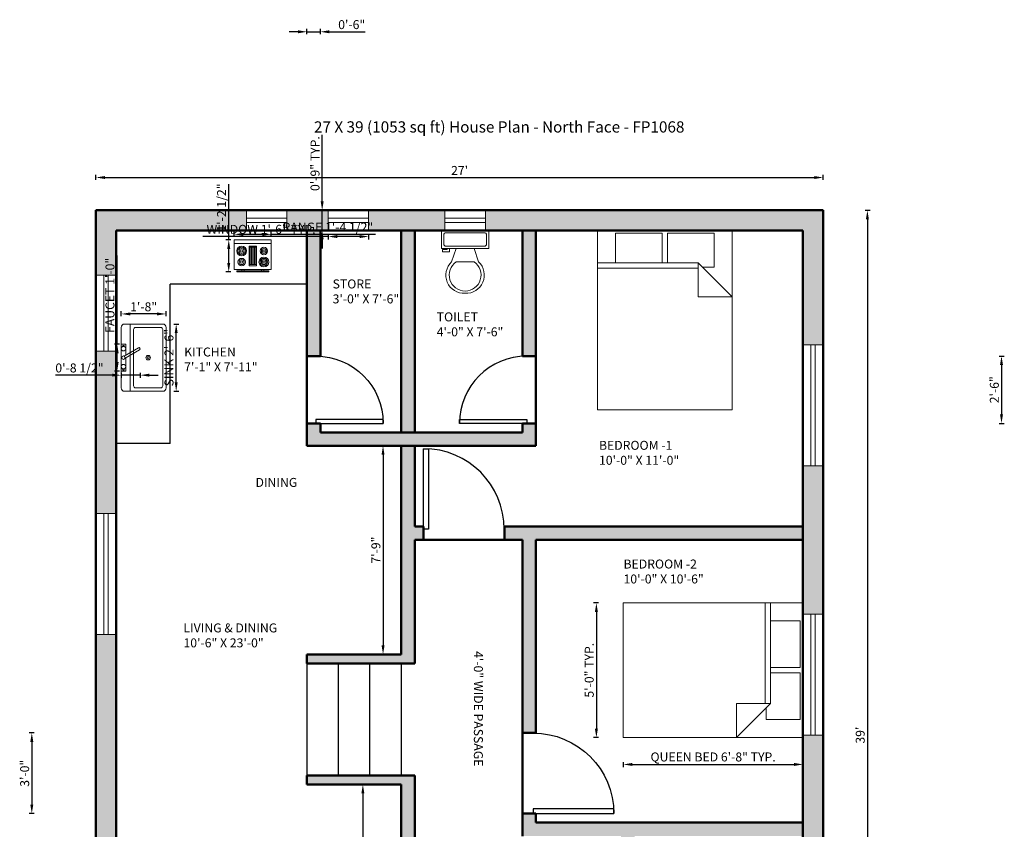
# Model space of a CAD drawing. Units: inches. Extents: x -33 to 405, y -509 to 99.
# Tile 2 of 2: x -33 to 405, y -262 to 99. Entities that reach past the tile are written whole.
import ezdxf

# ---------------------------------------------------------------- set-up
doc = ezdxf.new("R2010")
doc.units = ezdxf.units.IN
for name, color, linetype, lineweight in [('A-ANNO-DIMS', 2, 'Continuous', 18), ('A-ANNO-TEXT', 7, 'Continuous', 25), ('A-AREA-IDEN', 7, 'Continuous', 18), ('A-DOOR', 4, 'Continuous', 25), ('A-EQPM', 8, 'Continuous', 18), ('A-FLOR-CASE', 7, 'Continuous', 25), ('A-FLOR-FIXT', 8, 'Continuous', 18), ('A-FLOR-STRS', 7, 'Continuous', 25), ('A-FURN', 9, 'Continuous', 18), ('A-GLAZ', 6, 'Continuous', 18), ('A-WALL', 7, 'Continuous', 50), ('A-WALL-PATT', 251, 'Continuous', 13)]:
    doc.layers.add(name, color=color, linetype=linetype, lineweight=lineweight)
doc.styles.get("Standard").update_dxf_attribs({"font": 'arial.ttf'})
doc.dimstyles.new('ISO-25', dxfattribs={"dimtxt": 4, "dimasz": 4, "dimexe": 1.25, "dimexo": 0.625, "dimtad": 1, "dimlunit": 3, "dimtxsty": 'Standard', "dimcen": 2.5, "dimadec": 0, "dimazin": 0, "dimtfac": 1, "dimtmove": 0, "dimatfit": 3, "dimfxl": 1, "dimfxlon": 1, "dimarcsym": 0})

# ---------------------------------------------------------------- blocks, each defined once
blk = doc.blocks.new('*U4')
for p, q in [((0, 0), (0, -100)), ((750, 0), (750, -100))]:
    blk.add_line(p, q)
blk.add_lwpolyline([(0, 0), (0, 750), (43.75, 750), (43.75, 0)], close=True)
blk.add_arc((0, 0), 750, 0, 90)
blk = doc.blocks.new('*U2')
for p, q in [((9.5, -6), (9.5, -2)), ((-10, -8.5), (-8, -8.5)), ((-10, -9.5), (-10, -8.5)), ((-8, -8.5), (-8, -8)), ((-7, -8), (-7, -9.5)), ((-4, -8), (-6, -14)), ((4, -8), (6, -14)), ((-7, -9.5), (-10, -9.5)), ((4, -14), (-4, -14))]:
    blk.add_line(p, q)
blk.add_lwpolyline([(10.5, -8), (10.5, 0), (-10.5, 0), (-10.5, -8)], close=True)
for points in [[(-9.5, -2), (-9.5, -6)], [(8.5, -1), (-8.5, -1)], [(-8.5, -7), (8.5, -7)]]:
    blk.add_lwpolyline(points)
for centre, radius, start, end in [((-8.625, -1.875), 0.8839, 81.8699, 188.1301), ((8.625, -1.875), 0.8839, 351.8699, 98.1301), ((-8.625, -6.125), 0.8839, 171.869898, 278.1301), ((8.625, -6.125), 0.8839, 261.8699, 8.1301), ((-0.4772, -19.9188), 8.0953, 133.01722, 273.38), ((0.0374, -19.8731), 7.127, 124.50543, 269.7), ((-0.0373, -19.8731), 7.127, 270.3, 55.4946), ((0.4773, -19.9188), 8.0953, 266.62, 46.9828)]:
    blk.add_arc(centre, radius, start, end)
blk = doc.blocks.new('Sink-single - 30 in top')
blk.add_line((-15, -3.999996), (15, -3.999996))
for points in [[(-13.5, 0), (13.5, 0)], [(-15, -18.499996), (-15, -1.5)], [(15, -1.5), (15, -18.499996)], [(-13.5, -17.499996), (-13.5, -6.499996)], [(-12.5, -5.499996), (12.5, -5.499996)], [(13.5, -6.499996), (13.5, -17.499996)], [(13.5, -19.999996), (-13.5, -19.999996)], [(12.5, -18.499996), (-12.5, -18.499996)]]:
    blk.add_lwpolyline(points)
for radius in [1, 0.5]:
    blk.add_circle((0, -11.999996), radius)
for centre, radius, start, end in [((-13.5, -1.5), 1.5, 90, 180), ((13.5, -1.5), 1.5, 0, 90), ((-12.5, -6.499996), 1, 90, 180), ((12.5, -6.499996), 1, 0, 90), ((-12.5, -17.499996), 1, 180, 270), ((12.5, -17.499996), 1, 270, 0), ((-13.5, -18.499996), 1.5, 180, 270), ((13.5, -18.499996), 1.5, 270, 0)]:
    blk.add_arc(centre, radius, start, end)
blk = doc.blocks.new('Faucet - kit sink top')
for p, q in [((-5.5, -0.75), (-5.5, -1.25)), ((-4.94278, -0.75), (-5.5, -0.75)), ((-5.5, -1.25), (-4.94278, -1.25)), ((-0.14775, -1.7441), (3.56698, -8.1782)), ((4.43301, -7.6782), (0.71828, -1.2441)), ((4.94278, -0.75), (5.5, -0.75)), ((5.5, -1.25), (4.94278, -1.25)), ((5.5, -0.75), (5.5, -1.25))]:
    blk.add_line(p, q)
blk.add_lwpolyline([(-0.00587, -2), (-6, -2), (-6, 0), (6, 0), (6, -2), (1.15195, -2)])
for centre, radius in [((-4, -1), 1), ((4, -1), 1), ((0, -1), 0.75)]:
    blk.add_circle(centre, radius)
blk.add_arc((4, -7.9282), 0.5, 210, 30)
blk = doc.blocks.new('Range-Oven - 30 in top')
for p, q in [((0, -3), (30, -3)), ((12, -6), (18, -6)), ((13, -20), (13, -6)), ((14, -6), (14, -20)), ((15, -20), (15, -6)), ((16, -6), (16, -20)), ((17, -20), (17, -6)), ((18, -20), (12, -20)), ((6, -24), (6, -25)), ((8, -25), (8, -24)), ((22, -25), (22, -24)), ((24, -24), (24, -25))]:
    blk.add_line(p, q)
for points in [[(0, -24), (0, 0), (30, 0), (30, -24)], [(12, -21), (12, -5), (18, -5), (18, -21)], [(2, -26), (2, -25), (28, -25), (28, -26)]]:
    blk.add_lwpolyline(points, close=True)
for centre, radius in [((6, -9), 4), ((6, -9), 3), ((6, -9), 2), ((24, -9), 3), ((24, -9), 2), ((6, -18), 3), ((6, -9), 1), ((24, -18), 4), ((24, -18), 3), ((24, -9), 1), ((6, -18), 2), ((6, -18), 1), ((24, -18), 2), ((24, -18), 1)]:
    blk.add_circle(centre, radius)
blk = doc.blocks.new('Bed - Queen')
for p, q in [((0, -80.00003), (0, 0)), ((0, 0), (59.99999, 0)), ((59.99999, 0), (59.99999, -80.00003)), ((7.99999, -1.2), (28.79998, -1.2)), ((7.99999, -14.4), (7.99999, -1.2)), ((28.79998, -1.2), (28.79998, -14.4)), ((31.19999, -1.2), (51.99999, -1.2)), ((31.19999, -14.4), (31.19999, -1.2)), ((51.99999, -1.2), (51.99999, -16.4)), ((0, -14.4), (44.8, -14.4)), ((44.8, -16.8), (0, -16.8)), ((59.99999, -29.6), (44.8, -14.4)), ((44.8, -14.4), (44.8, -29.6)), ((51.99999, -16.4), (46.79936, -16.4)), ((44.8, -29.6), (59.99999, -29.6)), ((59.99999, -80.00003), (0, -80.00003))]:
    blk.add_line(p, q)
blk = doc.blocks.new('*D12')
at = {"layer": 'A-ANNO-DIMS', "color": 0, "lineweight": -2, "transparency": 16777216}
for p, q in [((128.59, -90.55), (129.84, -90.55)), ((128.59, -94.55), (128.59, -179.55)), ((128.59, -183.55), (129.84, -183.55))]:
    blk.add_line(p, q, dxfattribs=at)
at = {"layer": 'A-ANNO-DIMS', "color": 0, "transparency": 16777216}
for points in [[(127.92, -94.55), (129.25, -94.55), (128.59, -90.55)], [(127.92, -179.55), (129.25, -179.55), (128.59, -183.55)]]:
    blk.add_solid(points, dxfattribs=at)
at = {"layer": 'Defpoints', "color": 0, "transparency": 16777216}
for p in [(128.27, -90.55), (128.27, -183.55), (128.59, -183.55)]:
    blk.add_point(p, dxfattribs=at)
at = {"layer": 'A-ANNO-DIMS', "color": 0, "transparency": 16777216, "insert": (125.92, -137.05), "char_height": 4, "attachment_point": 5, "rotation": 90}
blk.add_mtext('7\'-9"', dxfattribs=at)
blk = doc.blocks.new('*D13')
at = {"layer": 'A-ANNO-DIMS', "color": 0, "lineweight": -2, "transparency": 16777216}
for p, q in [((120.59, -241.55), (118.34, -241.55)), ((119.59, -245.55), (119.59, -360.55)), ((120.59, -364.55), (118.34, -364.55))]:
    blk.add_line(p, q, dxfattribs=at)
at = {"layer": 'A-ANNO-DIMS', "color": 0, "transparency": 16777216}
for points in [[(118.92, -245.55), (120.26, -245.55), (119.59, -241.55)], [(118.92, -360.55), (120.26, -360.55), (119.59, -364.55)]]:
    blk.add_solid(points, dxfattribs=at)
at = {"layer": 'Defpoints', "color": 0, "transparency": 16777216}
for p in [(125.69, -241.55), (119.59, -364.55), (125.69, -364.55)]:
    blk.add_point(p, dxfattribs=at)
at = {"layer": 'A-ANNO-DIMS', "color": 0, "transparency": 16777216, "insert": (116.92, -303.05), "char_height": 4, "attachment_point": 5, "rotation": 90}
blk.add_mtext('10\'-3"', dxfattribs=at)
blk = doc.blocks.new('*D15')
at = {"layer": 'A-ANNO-DIMS', "color": 0, "lineweight": -2, "transparency": 16777216}
for p, q in [((0.69, 28.07), (0.69, 30.32)), ((4.69, 29.07), (320.69, 29.07)), ((324.69, 28.07), (324.69, 30.32))]:
    blk.add_line(p, q, dxfattribs=at)
at = {"layer": 'A-ANNO-DIMS', "color": 0, "transparency": 16777216}
for points in [[(4.69, 29.73), (4.69, 28.4), (0.69, 29.07)], [(320.69, 29.73), (320.69, 28.4), (324.69, 29.07)]]:
    blk.add_solid(points, dxfattribs=at)
at = {"layer": 'Defpoints', "color": 0, "transparency": 16777216}
for p in [(324.69, 29.07), (0.69, 14.45), (324.69, 14.45)]:
    blk.add_point(p, dxfattribs=at)
at = {"layer": 'A-ANNO-DIMS', "color": 0, "transparency": 16777216, "insert": (162.69, 31.7), "char_height": 4, "attachment_point": 5}
blk.add_mtext("27'", dxfattribs=at)
blk = doc.blocks.new('*D16')
at = {"layer": 'A-ANNO-DIMS', "color": 0, "lineweight": -2, "transparency": 16777216}
for p, q in [((343.39, 14.45), (345.64, 14.45)), ((344.39, 10.45), (344.39, -449.55)), ((343.39, -453.55), (345.64, -453.55))]:
    blk.add_line(p, q, dxfattribs=at)
at = {"layer": 'A-ANNO-DIMS', "color": 0, "transparency": 16777216}
for points in [[(343.72, 10.45), (345.06, 10.45), (344.39, 14.45)], [(343.72, -449.55), (345.06, -449.55), (344.39, -453.55)]]:
    blk.add_solid(points, dxfattribs=at)
at = {"layer": 'Defpoints', "color": 0, "transparency": 16777216}
for p in [(324.69, 14.45), (324.69, -453.55), (344.39, -453.55)]:
    blk.add_point(p, dxfattribs=at)
at = {"layer": 'A-ANNO-DIMS', "color": 0, "transparency": 16777216, "insert": (341.72, -219.55), "char_height": 4, "attachment_point": 5, "rotation": 90}
blk.add_mtext("39'", dxfattribs=at)
blk = doc.blocks.new('WIN-54IN')
for p, q in [((54, 5.5), (0, 5.5)), ((54, 3.5), (0, 3.5))]:
    blk.add_line(p, q)
blk.add_lwpolyline([(54, 9), (54, 0), (0, 0), (0, 9)], close=True)
blk = doc.blocks.new('WIN-18IN')
for p, q in [((3.5, 18), (3.5, 0)), ((5.5, 18), (5.5, 0))]:
    blk.add_line(p, q)
blk.add_lwpolyline([(9, 18), (9, 0), (0, 0), (0, 18)], close=True)
blk = doc.blocks.new('WIN-34IN')
for p, q in [((3.5, 34), (3.5, 0)), ((5.5, 34), (5.5, 0))]:
    blk.add_line(p, q)
blk.add_lwpolyline([(0, 34), (9, 34), (9, 0), (0, 0)], close=True)
blk = doc.blocks.new('*D22')
at = {"layer": 'A-ANNO-DIMS', "color": 0, "lineweight": -2, "transparency": 16777216}
for p, q in [((104.17, 2.75), (48.3, 2.75)), ((104.17, 3.75), (104.17, 1.5)), ((118.17, 2.75), (108.17, 2.75)), ((122.17, 3.75), (122.17, 1.5))]:
    blk.add_line(p, q, dxfattribs=at)
at = {"layer": 'A-ANNO-DIMS', "color": 0, "transparency": 16777216}
for points in [[(108.17, 3.42), (108.17, 2.08), (104.17, 2.75)], [(118.17, 3.42), (118.17, 2.08), (122.17, 2.75)]]:
    blk.add_solid(points, dxfattribs=at)
at = {"layer": 'Defpoints', "color": 0, "transparency": 16777216}
for p in [(104.17, 5.45), (122.17, 5.45), (104.17, 2.75)]:
    blk.add_point(p, dxfattribs=at)
at = {"layer": 'A-ANNO-DIMS', "color": 0, "transparency": 16777216, "insert": (74.23, 5.45), "char_height": 4, "attachment_point": 5}
blk.add_mtext('WINDOW 1\'-6" TYP.', dxfattribs=at)
blk = doc.blocks.new('*D23')
at = {"layer": 'A-ANNO-DIMS', "color": 0, "lineweight": -2, "transparency": 16777216}
for p, q in [((101.47, 18.45), (101.47, 48.08)), ((102.47, 14.45), (100.22, 14.45)), ((101.47, 5.45), (101.47, 14.45)), ((102.47, 5.45), (100.22, 5.45)), ((101.47, 1.45), (101.47, -2.55))]:
    blk.add_line(p, q, dxfattribs=at)
at = {"layer": 'A-ANNO-DIMS', "color": 0, "transparency": 16777216}
for points in [[(100.8, 18.45), (102.13, 18.45), (101.47, 14.45)], [(100.8, 1.45), (102.13, 1.45), (101.47, 5.45)]]:
    blk.add_solid(points, dxfattribs=at)
at = {"layer": 'Defpoints', "color": 0, "transparency": 16777216}
for p in [(101.47, 14.45), (104.17, 14.45), (104.17, 5.45)]:
    blk.add_point(p, dxfattribs=at)
at = {"layer": 'A-ANNO-DIMS', "color": 0, "transparency": 16777216, "insert": (98.8, 35.27), "char_height": 4, "attachment_point": 5, "rotation": 90}
blk.add_mtext('0\'-9" TYP.', dxfattribs=at)
blk = doc.blocks.new('*D26')
at = {"layer": 'A-ANNO-DIMS', "color": 0, "lineweight": -2, "transparency": 16777216}
for p, q in [((235.65, -231.62), (235.65, -233.87)), ((315.65, -231.62), (315.65, -233.87)), ((239.65, -232.62), (311.65, -232.62))]:
    blk.add_line(p, q, dxfattribs=at)
at = {"layer": 'A-ANNO-DIMS', "color": 0, "transparency": 16777216}
for points in [[(239.65, -231.95), (239.65, -233.29), (235.65, -232.62)], [(311.65, -231.95), (311.65, -233.29), (315.65, -232.62)]]:
    blk.add_solid(points, dxfattribs=at)
at = {"layer": 'Defpoints', "color": 0, "transparency": 16777216}
for p in [(235.65, -220.62), (315.65, -220.62), (315.65, -232.62)]:
    blk.add_point(p, dxfattribs=at)
at = {"layer": 'A-ANNO-DIMS', "color": 0, "transparency": 16777216, "insert": (275.65, -229.8), "char_height": 4, "attachment_point": 5}
blk.add_mtext('QUEEN BED 6\'-8" TYP.', dxfattribs=at)
blk = doc.blocks.new('*D27')
at = {"layer": 'A-ANNO-DIMS', "color": 0, "lineweight": -2, "transparency": 16777216}
for p, q in [((224.65, -160.62), (222.4, -160.62)), ((223.65, -164.62), (223.65, -216.62)), ((224.65, -220.62), (222.4, -220.62))]:
    blk.add_line(p, q, dxfattribs=at)
at = {"layer": 'A-ANNO-DIMS', "color": 0, "transparency": 16777216}
for points in [[(222.98, -164.62), (224.32, -164.62), (223.65, -160.62)], [(222.98, -216.62), (224.32, -216.62), (223.65, -220.62)]]:
    blk.add_solid(points, dxfattribs=at)
at = {"layer": 'Defpoints', "color": 0, "transparency": 16777216}
for p in [(235.65, -160.62), (223.65, -220.62), (235.65, -220.62)]:
    blk.add_point(p, dxfattribs=at)
at = {"layer": 'A-ANNO-DIMS', "color": 0, "transparency": 16777216, "insert": (220.98, -190.62), "char_height": 4, "attachment_point": 5, "rotation": 90}
blk.add_mtext('5\'-0" TYP.', dxfattribs=at)
blk = doc.blocks.new('*D28')
at = {"layer": 'A-ANNO-DIMS', "color": 0, "lineweight": -2, "transparency": 16777216}
for p, q in [((35.42, -36.26), (37.67, -36.26)), ((36.42, -62.26), (36.42, -40.26)), ((35.42, -66.26), (37.67, -66.26))]:
    blk.add_line(p, q, dxfattribs=at)
at = {"layer": 'A-ANNO-DIMS', "color": 0, "transparency": 16777216}
for points in [[(35.76, -40.26), (37.09, -40.26), (36.42, -36.26)], [(35.76, -62.26), (37.09, -62.26), (36.42, -66.26)]]:
    blk.add_solid(points, dxfattribs=at)
at = {"layer": 'Defpoints', "color": 0, "transparency": 16777216}
for p in [(31.92, -36.26), (36.42, -36.26), (31.92, -66.26)]:
    blk.add_point(p, dxfattribs=at)
at = {"layer": 'A-ANNO-DIMS', "color": 0, "transparency": 16777216, "insert": (33.73, -51.26), "char_height": 4, "attachment_point": 5, "rotation": 90}
blk.add_mtext('SINK 2\'-6"', dxfattribs=at)
blk = doc.blocks.new('*D29')
at = {"layer": 'A-ANNO-DIMS', "color": 0, "lineweight": -2, "transparency": 16777216}
for p, q in [((11.92, -32.76), (11.92, -30.51)), ((31.92, -32.76), (31.92, -30.51)), ((27.92, -31.76), (15.92, -31.76))]:
    blk.add_line(p, q, dxfattribs=at)
at = {"layer": 'A-ANNO-DIMS', "color": 0, "transparency": 16777216}
for points in [[(15.92, -31.09), (15.92, -32.42), (11.92, -31.76)], [(27.92, -31.09), (27.92, -32.42), (31.92, -31.76)]]:
    blk.add_solid(points, dxfattribs=at)
at = {"layer": 'Defpoints', "color": 0, "transparency": 16777216}
for p in [(11.92, -31.76), (11.92, -36.26), (31.92, -36.26)]:
    blk.add_point(p, dxfattribs=at)
at = {"layer": 'A-ANNO-DIMS', "color": 0, "transparency": 16777216, "insert": (21.92, -29.09), "char_height": 4, "attachment_point": 5}
blk.add_mtext('1\'-8"', dxfattribs=at)
blk = doc.blocks.new('*D30')
at = {"layer": 'A-ANNO-DIMS', "color": 0, "lineweight": -2, "transparency": 16777216}
for p, q in [((10.12, -45.26), (10.12, -5.69)), ((11.12, -45.26), (8.87, -45.26)), ((10.12, -53.26), (10.12, -49.26)), ((11.12, -57.26), (8.87, -57.26))]:
    blk.add_line(p, q, dxfattribs=at)
at = {"layer": 'A-ANNO-DIMS', "color": 0, "transparency": 16777216}
for points in [[(9.46, -49.26), (10.79, -49.26), (10.12, -45.26)], [(9.46, -53.26), (10.79, -53.26), (10.12, -57.26)]]:
    blk.add_solid(points, dxfattribs=at)
at = {"layer": 'Defpoints', "color": 0, "transparency": 16777216}
for p in [(10.12, -45.26), (11.92, -45.26), (11.92, -57.26)]:
    blk.add_point(p, dxfattribs=at)
at = {"layer": 'A-ANNO-DIMS', "color": 0, "transparency": 16777216, "insert": (7.43, -23.47), "char_height": 4, "attachment_point": 5, "rotation": 90}
blk.add_mtext('FAUCET 1\'-0"', dxfattribs=at)
blk = doc.blocks.new('*D31')
at = {"layer": 'A-ANNO-DIMS', "color": 0, "lineweight": -2, "transparency": 16777216}
for p, q in [((7.92, -59.06), (-17.28, -59.06)), ((11.92, -58.06), (11.92, -60.31)), ((20.42, -59.06), (11.92, -59.06)), ((20.42, -58.06), (20.42, -60.31)), ((24.42, -59.06), (28.42, -59.06))]:
    blk.add_line(p, q, dxfattribs=at)
at = {"layer": 'A-ANNO-DIMS', "color": 0, "transparency": 16777216}
for points in [[(7.92, -58.39), (7.92, -59.72), (11.92, -59.06)], [(24.42, -58.39), (24.42, -59.72), (20.42, -59.06)]]:
    blk.add_solid(points, dxfattribs=at)
at = {"layer": 'Defpoints', "color": 0, "transparency": 16777216}
for p in [(11.92, -57.26), (11.92, -59.06), (20.42, -57.26)]:
    blk.add_point(p, dxfattribs=at)
at = {"layer": 'A-ANNO-DIMS', "color": 0, "transparency": 16777216, "insert": (-6.68, -56.36), "char_height": 4, "attachment_point": 5}
blk.add_mtext('0\'-8 1/2"', dxfattribs=at)
blk = doc.blocks.new('*D32')
at = {"layer": 'A-ANNO-DIMS', "color": 0, "lineweight": -2, "transparency": 16777216}
for p, q in [((62.31, 2.74), (62.31, 4.99)), ((78.8, 2.74), (78.8, 4.99)), ((66.31, 3.74), (74.8, 3.74)), ((78.8, 3.74), (125.22, 3.74))]:
    blk.add_line(p, q, dxfattribs=at)
at = {"layer": 'A-ANNO-DIMS', "color": 0, "transparency": 16777216}
for points in [[(66.31, 4.41), (66.31, 3.07), (62.31, 3.74)], [(74.8, 4.41), (74.8, 3.07), (78.8, 3.74)]]:
    blk.add_solid(points, dxfattribs=at)
at = {"layer": 'Defpoints', "color": 0, "transparency": 16777216}
for p in [(62.31, 1.27), (78.8, 3.74), (78.8, 1.27)]:
    blk.add_point(p, dxfattribs=at)
at = {"layer": 'A-ANNO-DIMS', "color": 0, "transparency": 16777216, "insert": (104.01, 6.43), "char_height": 4, "attachment_point": 5}
blk.add_mtext('RANGE 1\'-4 1/2"', dxfattribs=at)
blk = doc.blocks.new('*D33')
at = {"layer": 'A-ANNO-DIMS', "color": 0, "lineweight": -2, "transparency": 16777216}
for p, q in [((59.83, 1.27), (59.83, 26.09)), ((60.83, 1.27), (58.58, 1.27)), ((59.83, -9.03), (59.83, -2.73)), ((60.83, -13.03), (58.58, -13.03))]:
    blk.add_line(p, q, dxfattribs=at)
at = {"layer": 'A-ANNO-DIMS', "color": 0, "transparency": 16777216}
for points in [[(59.17, -2.73), (60.5, -2.73), (59.83, 1.27)], [(59.17, -9.03), (60.5, -9.03), (59.83, -13.03)]]:
    blk.add_solid(points, dxfattribs=at)
at = {"layer": 'Defpoints', "color": 0, "transparency": 16777216}
for p in [(59.83, 1.27), (62.31, 1.27), (62.31, -13.03)]:
    blk.add_point(p, dxfattribs=at)
at = {"layer": 'A-ANNO-DIMS', "color": 0, "transparency": 16777216, "insert": (57.14, 15.68), "char_height": 4, "attachment_point": 5, "rotation": 90}
blk.add_mtext('1\'-2 1/2"', dxfattribs=at)
blk = doc.blocks.new('*D37')
at = {"layer": 'A-ANNO-DIMS', "color": 0, "lineweight": -2, "transparency": 16777216}
for p, q in [((9.69, -505.21), (9.69, -507.46)), ((13.69, -506.21), (29.69, -506.21)), ((33.69, -505.21), (33.69, -507.46))]:
    blk.add_line(p, q, dxfattribs=at)
at = {"layer": 'A-ANNO-DIMS', "color": 0, "transparency": 16777216}
for points in [[(13.69, -505.54), (13.69, -506.87), (9.69, -506.21)], [(29.69, -505.54), (29.69, -506.87), (33.69, -506.21)]]:
    blk.add_solid(points, dxfattribs=at)
at = {"layer": 'Defpoints', "color": 0, "transparency": 16777216}
for p in [(9.69, -89.55), (33.69, -89.55), (33.69, -506.21)]:
    blk.add_point(p, dxfattribs=at)
at = {"layer": 'A-ANNO-DIMS', "color": 0, "transparency": 16777216, "insert": (21.69, -503.54), "char_height": 4, "attachment_point": 5}
blk.add_mtext('2\'-0"', dxfattribs=at)
blk = doc.blocks.new('*D38')
at = {"layer": 'A-ANNO-DIMS', "color": 0, "lineweight": -2, "transparency": 16777216}
for p, q in [((403.15, -50.55), (405.4, -50.55)), ((404.15, -54.55), (404.15, -76.55)), ((403.15, -80.55), (405.4, -80.55))]:
    blk.add_line(p, q, dxfattribs=at)
at = {"layer": 'A-ANNO-DIMS', "color": 0, "transparency": 16777216}
for points in [[(403.48, -54.55), (404.82, -54.55), (404.15, -50.55)], [(403.48, -76.55), (404.82, -76.55), (404.15, -80.55)]]:
    blk.add_solid(points, dxfattribs=at)
at = {"layer": 'Defpoints', "color": 0, "transparency": 16777216}
for p in [(94.69, -50.55), (94.69, -80.55), (404.15, -80.55)]:
    blk.add_point(p, dxfattribs=at)
at = {"layer": 'A-ANNO-DIMS', "color": 0, "transparency": 16777216, "insert": (401.48, -65.55), "char_height": 4, "attachment_point": 5, "rotation": 90}
blk.add_mtext('2\'-6"', dxfattribs=at)
blk = doc.blocks.new('*D39')
at = {"layer": 'A-ANNO-DIMS', "color": 0, "lineweight": -2, "transparency": 16777216}
for p, q in [((90.69, 94.05), (86.69, 94.05)), ((94.69, 93.05), (94.69, 95.3)), ((94.69, 94.05), (100.69, 94.05)), ((100.69, 93.05), (100.69, 95.3)), ((104.69, 94.05), (120.57, 94.05))]:
    blk.add_line(p, q, dxfattribs=at)
at = {"layer": 'A-ANNO-DIMS', "color": 0, "transparency": 16777216}
for points in [[(90.69, 94.72), (90.69, 93.38), (94.69, 94.05)], [(104.69, 94.72), (104.69, 93.38), (100.69, 94.05)]]:
    blk.add_solid(points, dxfattribs=at)
at = {"layer": 'Defpoints', "color": 0, "transparency": 16777216}
for p in [(100.69, 94.05), (94.69, 5.45), (100.69, 5.45)]:
    blk.add_point(p, dxfattribs=at)
at = {"layer": 'A-ANNO-DIMS', "color": 0, "transparency": 16777216, "insert": (114.63, 96.72), "char_height": 4, "attachment_point": 5}
blk.add_mtext('0\'-6"', dxfattribs=at)
blk = doc.blocks.new('*D40')
at = {"layer": 'A-ANNO-DIMS', "color": 0, "lineweight": -2, "transparency": 16777216}
for p, q in [((-26.91, -218.55), (-29.16, -218.55)), ((-27.91, -222.55), (-27.91, -250.55)), ((-26.91, -254.55), (-29.16, -254.55))]:
    blk.add_line(p, q, dxfattribs=at)
at = {"layer": 'A-ANNO-DIMS', "color": 0, "transparency": 16777216}
for points in [[(-28.58, -222.55), (-27.25, -222.55), (-27.91, -218.55)], [(-28.58, -250.55), (-27.25, -250.55), (-27.91, -254.55)]]:
    blk.add_solid(points, dxfattribs=at)
at = {"layer": 'Defpoints', "color": 0, "transparency": 16777216}
for p in [(190.69, -218.55), (-27.91, -254.55), (190.69, -254.55)]:
    blk.add_point(p, dxfattribs=at)
at = {"layer": 'A-ANNO-DIMS', "color": 0, "transparency": 16777216, "insert": (-30.58, -236.55), "char_height": 4, "attachment_point": 5, "rotation": 90}
blk.add_mtext('3\'-0"', dxfattribs=at)

msp = doc.modelspace()

# ---------------------------------------------------------------- hatches: boundary and pattern name
at = {"layer": 'A-WALL-PATT'}
h = msp.add_hatch(color=256, dxfattribs=at)
h.dxf.hatch_style = 1
h.paths.add_polyline_path([(67.714, 14.451), (0.686, 14.451), (0.686, -14.411), (9.686, -14.411), (9.686, 5.451), (67.714, 5.451)])
h.paths.add_polyline_path([(324.686, 14.451), (174.189, 14.451), (174.189, 5.451), (175.65, 5.451), (196.686, 5.451), (315.686, 5.451), (315.686, -45.53), (324.686, -45.53)])
h.paths.add_polyline_path([(156.189, 14.451), (122.165, 14.451), (122.165, 5.451), (156.189, 5.451)])
h.paths.add_polyline_path([(104.165, 14.451), (85.714, 14.451), (85.714, 5.451), (94.686, 5.451), (104.165, 5.451)])
h = msp.add_hatch(color=256, dxfattribs=at)
h.dxf.hatch_style = 1
h.paths.add_polyline_path([(9.686, -48.411), (0.686, -48.411), (0.686, -120.696), (9.686, -120.696)])
h.paths.add_polyline_path([(100.686, 5.451), (94.686, 5.451), (94.686, -50.549), (100.686, -50.549)])
h.paths.add_polyline_path([(142.686, 5.451), (136.686, 5.451), (136.686, -84.549), (142.686, -84.549)])
h.paths.add_polyline_path([(196.686, 5.451), (190.686, 5.451), (190.686, -50.609), (190.777, -50.609, -0.0158204), (192.678, -50.549), (196.686, -50.549)])
h.paths.add_polyline_path([(196.686, -80.609), (192.678, -80.609), (190.686, -80.609), (190.686, -84.549), (100.686, -84.549), (100.686, -80.549), (98.685, -80.549), (94.686, -80.549), (94.686, -90.549), (196.686, -90.549)])
h.paths.add_polyline_path([(324.686, -99.53), (315.686, -99.53), (315.686, -165.584), (324.686, -165.584)])
h.paths.add_polyline_path([(315.686, -126.549), (182.686, -126.549), (182.686, -132.549), (190.686, -132.549), (190.686, -218.549), (196.686, -218.549), (196.686, -132.549), (315.686, -132.549)])
h.paths.add_polyline_path([(142.686, -90.549), (136.686, -90.549), (136.686, -183.549), (94.686, -183.549), (94.686, -187.549), (142.686, -187.549), (142.686, -132.549), (146.686, -132.549), (146.686, -127.759), (146.686, -126.549), (142.686, -126.549)])
h.paths.add_polyline_path([(142.686, -237.549), (94.686, -237.549), (94.686, -241.549), (136.686, -241.549), (136.686, -364.549), (9.686, -364.549), (9.686, -370.549), (136.686, -370.549), (150.686, -370.549), (150.686, -364.549), (142.686, -364.549)])
h.paths.add_polyline_path([(196.686, -312.549), (190.686, -312.549), (190.686, -444.549), (196.686, -444.549)])
h.paths.add_polyline_path([(190.686, -364.549), (186.686, -364.549), (186.686, -365.752), (186.686, -370.549), (190.686, -370.549)])
h.paths.add_polyline_path([(315.686, -312.549), (240.686, -312.549), (240.686, -298.549), (234.686, -298.549), (234.686, -312.549), (230.9, -312.549), (230.9, -317.111, -0.0105112), (230.87, -318.549), (234.686, -318.549), (240.686, -318.549), (315.686, -318.549)])
h.paths.add_polyline_path([(315.686, -258.549), (196.686, -258.549), (196.686, -254.549), (195.477, -254.549), (190.686, -254.549), (190.686, -264.549), (315.686, -264.549)])
h.paths.add_polyline_path([(240.686, -264.549), (234.686, -264.549), (234.686, -268.549), (238.649, -268.549), (240.686, -268.549)])
h.paths.add_polyline_path([(324.686, -296.335), (315.686, -296.335), (315.686, -444.549), (277.309, -444.549), (277.309, -453.549), (324.686, -453.549)])
h.paths.add_polyline_path([(324.686, -219.584), (315.686, -219.584), (315.686, -278.335), (324.686, -278.335)])
h.paths.add_polyline_path([(9.686, -174.696), (0.686, -174.696), (0.686, -292.323), (9.686, -292.323)])
h.paths.add_polyline_path([(9.686, -364.549), (9.686, -346.323), (0.686, -346.323), (0.686, -389.536), (9.686, -389.536), (9.686, -370.549)])
h.paths.add_polyline_path([(139.686, -444.549), (9.686, -444.549), (9.686, -423.536), (0.686, -423.536), (0.686, -453.549), (139.686, -453.549)])
h.paths.add_polyline_path([(223.309, -444.549), (181.686, -444.549), (181.686, -447.962), (181.686, -453.549), (223.309, -453.549)])

# ---------------------------------------------------------------- linework, layer by layer
at = {"layer": 'A-FLOR-CASE'}
for p, q in [((94.686, -18.549), (33.686, -18.549)), ((33.686, -89.549), (33.686, -18.549)), ((33.686, -89.549), (9.686, -89.549))]:
    msp.add_line(p, q, dxfattribs=at)
at = {"layer": 'A-FLOR-STRS'}
for p, q in [((94.686, -187.549), (94.686, -237.549)), ((108.598, -187.549), (108.598, -237.549)), ((122.511, -187.549), (122.511, -237.549)), ((136.686, -187.549), (136.686, -237.549))]:
    msp.add_line(p, q, dxfattribs=at)
at = {"layer": 'A-WALL'}
for p, q in [((0.686, 14.451), (324.686, 14.451)), ((0.686, -453.549), (0.686, 14.451)), ((324.686, 14.451), (324.686, -453.549)), ((9.686, 5.451), (94.686, 5.451)), ((9.686, -370.549), (9.686, 5.451)), ((94.686, -90.549), (94.686, 5.451)), ((94.686, 5.451), (196.686, 5.451)), ((100.686, -50.549), (100.686, 5.451)), ((136.686, -84.549), (136.686, 5.451)), ((142.686, -84.549), (142.686, 5.451)), ((190.686, -50.609), (190.686, 5.451)), ((196.686, 5.451), (315.686, 5.451)), ((196.686, -90.549), (196.686, 5.451)), ((315.686, 5.451), (315.686, -444.549)), ((100.686, -50.549), (94.686, -50.549)), ((190.686, -50.609), (196.686, -50.609)), ((100.686, -80.549), (94.686, -80.549)), ((100.686, -84.549), (100.686, -80.549)), ((190.686, -84.549), (190.686, -80.609)), ((190.686, -84.549), (190.686, -80.609)), ((190.686, -80.609), (196.686, -80.609)), ((196.686, -80.609), (196.686, -80.609)), ((100.686, -84.549), (190.686, -84.549)), ((94.686, -90.549), (196.686, -90.549)), ((136.686, -183.549), (136.686, -90.549)), ((142.686, -126.549), (142.686, -90.549)), ((142.686, -126.549), (146.686, -126.549)), ((146.686, -126.549), (146.686, -132.549)), ((182.686, -126.549), (182.686, -132.549)), ((182.686, -126.549), (315.686, -126.549)), ((142.686, -132.549), (190.686, -132.549)), ((142.686, -187.549), (142.686, -132.549)), ((190.686, -264.549), (190.686, -132.549)), ((196.686, -132.549), (315.686, -132.549)), ((196.686, -218.549), (196.686, -132.549)), ((136.686, -183.549), (94.686, -183.549)), ((94.686, -183.549), (94.686, -187.549)), ((142.686, -187.549), (94.686, -187.549)), ((196.686, -218.549), (190.686, -218.549)), ((94.686, -237.549), (142.686, -237.549)), ((94.686, -241.549), (94.686, -237.549)), ((142.686, -364.549), (142.686, -237.549)), ((94.686, -241.549), (136.686, -241.549)), ((136.686, -364.549), (136.686, -241.549)), ((196.686, -254.549), (190.686, -254.549)), ((196.686, -258.549), (196.686, -254.549)), ((196.686, -258.549), (315.686, -258.549))]:
    msp.add_line(p, q, dxfattribs=at)

# ---------------------------------------------------------------- block references
at = {"layer": 'A-DOOR'}
for p, xscale, yscale, zscale, rotation in [((98.685, -80.549), -0.0399961114547442, 0.0399961114547442, 0.0399961114547442, 270), ((192.678, -80.609), 0.0400802120255589, 0.0400802120255589, 0.0400802120255589, 89.99999999999999), ((195.477, -254.549), -0.0479093764917697, 0.0479093764917697, 0.0479093764917697, 270)]:
    msp.add_blockref('*U4', p, dxfattribs=dict(at, xscale=xscale, yscale=yscale, zscale=zscale, rotation=rotation))
at = {"layer": 'A-DOOR', "xscale": 0.0478989333779261, "yscale": 0.0478989333779261, "zscale": 0.0478989333779261}
msp.add_blockref('*U4', (146.686, -127.759), dxfattribs=at)
at = {"layer": 'A-EQPM', "xscale": 0.5497472873966894, "yscale": 0.5497472873966894, "zscale": 0.5497472873966894}
msp.add_blockref('Range-Oven - 30 in top', (62.307, 1.266), dxfattribs=at)
at = {"layer": 'A-FLOR-FIXT'}
msp.add_blockref('*U2', (165.15, 5.451), dxfattribs=at)
at = {"layer": 'A-FLOR-FIXT', "rotation": 90}
for name in ['Sink-single - 30 in top', 'Faucet - kit sink top']:
    msp.add_blockref(name, (11.924, -51.256), dxfattribs=at)
at = {"layer": 'A-FURN'}
msp.add_blockref('Bed - Queen', (224.157, 5.451), dxfattribs=at)
at = {"layer": 'A-FURN', "rotation": 270}
msp.add_blockref('Bed - Queen', (315.65, -160.62), dxfattribs=at)
at = {"layer": 'A-GLAZ'}
for name, p, rotation in [('WIN-18IN', (85.714, 5.451), 89.99999999999999), ('WIN-18IN', (122.165, 5.451), 89.99999999999994), ('WIN-18IN', (174.189, 5.451), 90.00000000000003), ('WIN-54IN', (324.686, -99.53), 90.00000000000018), ('WIN-54IN', (9.686, -174.696), 90.00000000000018), ('WIN-54IN', (324.686, -219.584), 90.00000000000018)]:
    msp.add_blockref(name, p, dxfattribs=dict(at, rotation=rotation))
msp.add_blockref('WIN-34IN', (0.686, -48.411), dxfattribs=at)

# ---------------------------------------------------------------- texts
at = {"layer": 'A-ANNO-TEXT', "insert": (97.805, 54.127), "char_height": 5, "attachment_point": 1}
msp.add_mtext_dynamic_manual_height_columns('27 X 39 (1053 sq ft) House Plan - North Face - FP1068', width=328.4867, gutter_width=12.5, heights=[0], dxfattribs=at)
at = {"layer": 'A-AREA-IDEN', "char_height": 4, "attachment_point": 1}
for s, width, insert in [('STORE\\P3\'-0" X 7\'-6"', 31.62533, (106.118, -16.385)), ('TOILET\\P4\'-0" X 7\'-6"', 30.37318, (152.509, -31.075)), ('KITCHEN\\P7\'-1" X 7\'-11"', 42.87394, (39.968, -46.721)), ('BEDROOM -1\\P10\'-0" X 11\'-0"', 67.03015, (224.808, -88.339)), ('DINING', 26.90489, (71.766, -104.874)), ('BEDROOM -2\\P10\'-0" X 10\'-6"', 40.7629, (235.741, -141.261)), ('LIVING & DINING\\P10\'-6" X 23\'-0"', 53.80695, (39.664, -169.751))]:
    msp.add_mtext_dynamic_manual_height_columns(s, width=width, gutter_width=12.5, heights=[0], dxfattribs=dict(at, insert=insert))
at = {"layer": 'A-AREA-IDEN', "insert": (173.066, -182.081), "char_height": 4, "attachment_point": 1, "rotation": 270}
msp.add_mtext_dynamic_manual_height_columns('4\'-0" WIDE PASSAGE', width=81.23666, gutter_width=12.5, heights=[0], dxfattribs=at)

# ---------------------------------------------------------------- dimensions: what is measured, and where the dimension line sits
at = {"layer": 'A-ANNO-DIMS'}
for base, p1, p2, override, picture, middle in [((100.686, 94.051), (94.686, 5.451), (100.686, 5.451), {"dimdec": 1, "dimlfac": 1, "dimrnd": 0, "dimzin": 1, "dimdsep": 46, "dimlunit": 4, "dimfrac": 2}, '*D39', (114.627, 96.718)), ((324.686, 29.068), (0.686, 14.451), (324.686, 14.451), {"dimclrd": 0, "dimclre": 0, "dimclrt": 0}, '*D15', (162.686, 31.701)), ((33.686, -506.205), (9.686, -89.549), (33.686, -89.549), {"dimdec": 1, "dimlfac": 1, "dimrnd": 0, "dimzin": 1, "dimdsep": 46, "dimlunit": 4, "dimfrac": 2}, '*D37', (21.686, -503.538))]:
    dim = msp.add_linear_dim(base=base, p1=p1, p2=p2, dimstyle='ISO-25', override=override, dxfattribs=at)
    dim.commit()
    dim.dimension.update_dxf_attribs({"geometry": picture, "text_midpoint": middle})
for base, p1, p2, angle, text, picture, middle in [((101.465, 14.451), (104.165, 5.451), (104.165, 14.451), 90, '<> TYP.', '*D23', (98.798, 35.267)), ((104.165, 2.751), (122.165, 5.451), (104.165, 5.451), 180, 'WINDOW <> TYP.', '*D22', (74.232, 5.445)), ((10.124, -45.256), (11.924, -57.256), (11.924, -45.256), 90, 'FAUCET <>', '*D30', (7.431, -23.475)), ((36.424, -36.256), (31.924, -66.256), (31.924, -36.256), 90, 'SINK <>', '*D28', (33.731, -51.256)), ((223.65, -220.62), (235.65, -160.62), (235.65, -220.62), 270, '<> TYP.', '*D27', (220.983, -190.62))]:
    dim = msp.add_linear_dim(base=base, p1=p1, p2=p2, angle=angle, text=text, dimstyle='ISO-25', override={"dimdec": 1, "dimlfac": 1, "dimrnd": 0, "dimzin": 1, "dimdsep": 46, "dimlunit": 4, "dimfrac": 2}, dxfattribs=at)
    dim.commit()
    dim.dimension.update_dxf_attribs({"geometry": picture, "text_midpoint": middle})
for base, p1, p2, angle, override, picture, middle in [((59.833, 1.266), (62.307, -13.027), (62.307, 1.266), 90, {"dimdec": 1, "dimlfac": 1, "dimrnd": 0, "dimzin": 1, "dimdsep": 46, "dimlunit": 4, "dimfrac": 2}, '*D33', (57.139, 15.679)), ((344.391, -453.549), (324.686, 14.451), (324.686, -453.549), 90, {"dimclrd": 0, "dimclre": 0, "dimclrt": 0}, '*D16', (341.723, -219.549)), ((11.924, -31.756), (31.924, -36.256), (11.924, -36.256), 180, {"dimdec": 1, "dimlfac": 1, "dimrnd": 0, "dimzin": 1, "dimdsep": 46, "dimlunit": 4, "dimfrac": 2}, '*D29', (21.924, -29.088)), ((11.924, -59.056), (20.424, -57.256), (11.924, -57.256), 180, {"dimdec": 1, "dimlfac": 1, "dimrnd": 0, "dimzin": 1, "dimdsep": 46, "dimlunit": 4, "dimfrac": 2}, '*D31', (-6.677, -56.362)), ((404.151, -80.549), (94.686, -50.549), (94.686, -80.549), 90, {"dimdec": 1, "dimlfac": 1, "dimrnd": 0, "dimzin": 1, "dimdsep": 46, "dimlunit": 4, "dimfrac": 2}, '*D38', (401.484, -65.549)), ((128.586, -183.549), (128.267, -90.549), (128.267, -183.549), 90, {"dimclrd": 0, "dimclre": 0, "dimclrt": 0}, '*D12', (125.919, -137.049)), ((-27.914, -254.549), (190.686, -218.549), (190.686, -254.549), 90, {"dimdec": 1, "dimlfac": 1, "dimrnd": 0, "dimzin": 1, "dimdsep": 46, "dimlunit": 4, "dimfrac": 2}, '*D40', (-30.583, -236.549)), ((119.588, -364.549), (125.691, -241.549), (125.691, -364.549), 90, {"dimclrd": 0, "dimclre": 0, "dimclrt": 0}, '*D13', (116.92, -303.049))]:
    dim = msp.add_linear_dim(base=base, p1=p1, p2=p2, angle=angle, dimstyle='ISO-25', override=override, dxfattribs=at)
    dim.commit()
    dim.dimension.update_dxf_attribs({"geometry": picture, "text_midpoint": middle})
for base, p1, p2, text, picture, middle in [((78.799, 3.74), (62.307, 1.266), (78.799, 1.266), 'RANGE <>', '*D32', (104.009, 6.433)), ((315.65, -232.62), (235.65, -220.62), (315.65, -220.62), 'QUEEN BED <> TYP.', '*D26', (275.65, -229.804))]:
    dim = msp.add_linear_dim(base=base, p1=p1, p2=p2, text=text, dimstyle='ISO-25', override={"dimdec": 1, "dimlfac": 1, "dimrnd": 0, "dimzin": 1, "dimdsep": 46, "dimlunit": 4, "dimfrac": 2}, dxfattribs=at)
    dim.commit()
    dim.dimension.update_dxf_attribs({"geometry": picture, "text_midpoint": middle})

doc.saveas('drawing.dxf')
